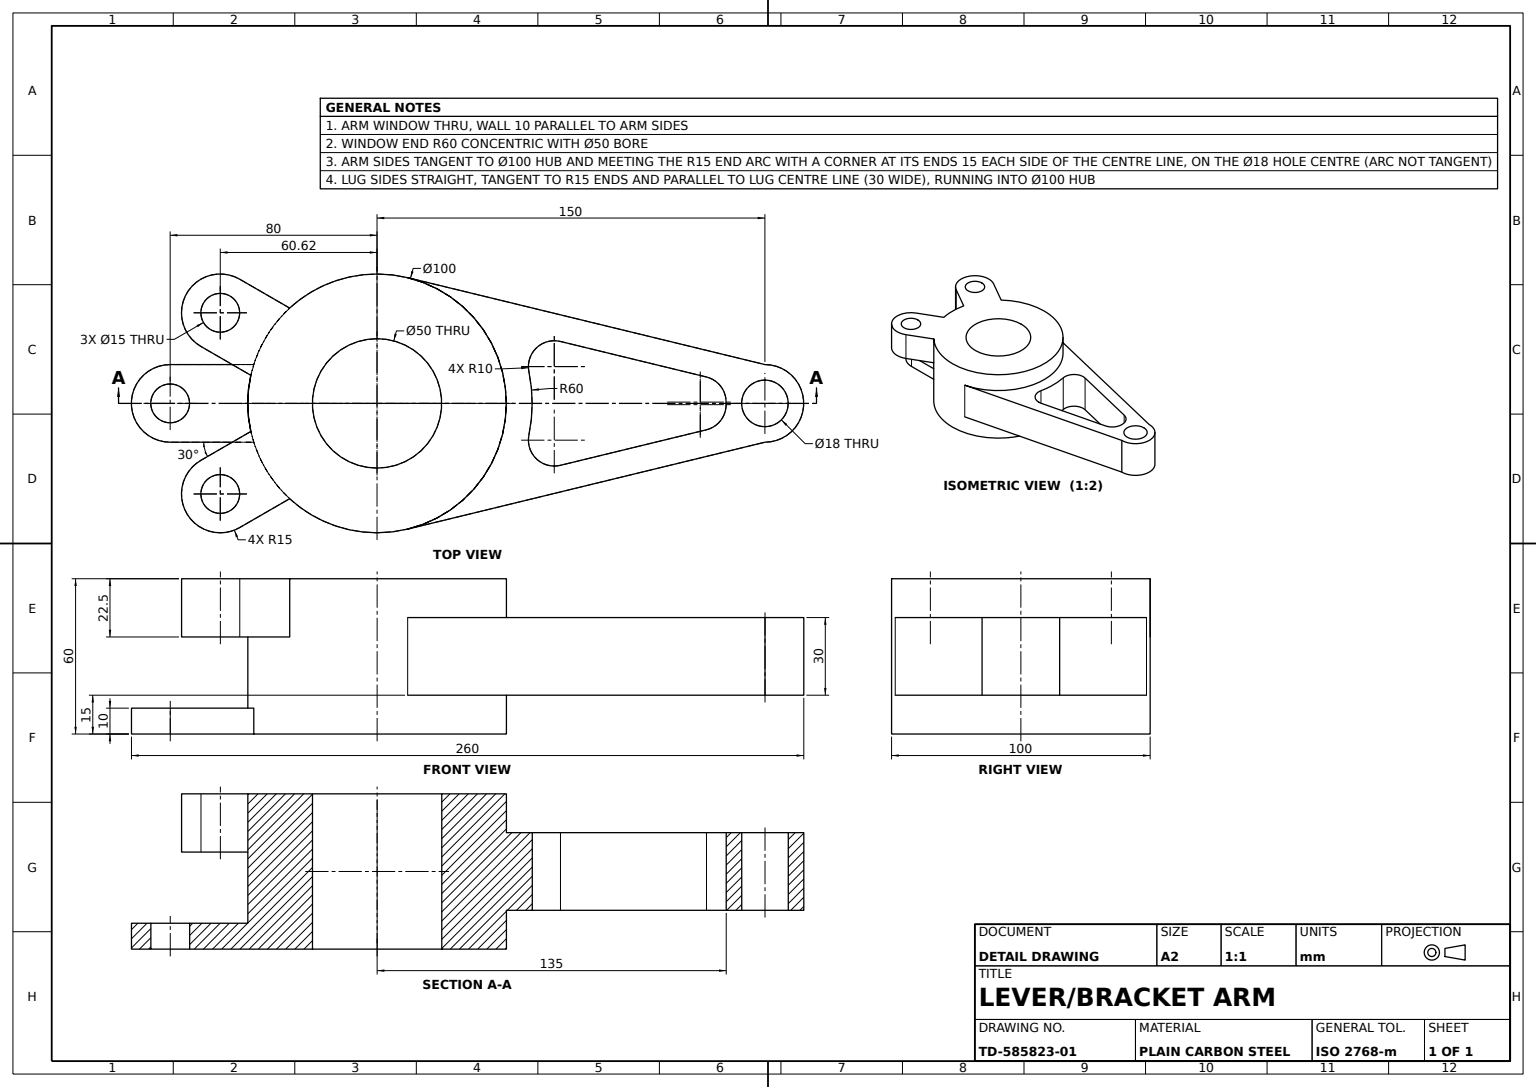
SolidWorks part; units mm, degrees
material "Plain Carbon Steel"
ref_plane "Front Plane" through (0, 0, 0) normal (0, 0, 1) x (1, 0, 0)
ref_plane "Top Plane" through (0, 0, 0) normal (0, 1, 0) x (1, 0, 0)
ref_plane "Right Plane" through (0, 0, 0) normal (1, 0, 0) x (0, 0, -1)
sketch "Hub Sketch" plane through (0, 0, 0) normal (0, 1, 0) x (1, 0, 0)
  circle A0 centre (0, 0) radius 25
  circle A1 centre (0, 0) radius 50
  dimension "D1" = 50
  dimension "D2" = 100
extrude "Hub Ø100 Bore Ø50" add sketch "Hub Sketch" along normal blind 60
ref_plane "Plane1" through (0, 30, 0) normal (0, 1, 0) x (1, 0, 0)
sketch "Lever Arm Sketch" plane through (0, 30, 0) normal (0, 1, 0) x (1, 0, 0)
  line L0 (0, 0) -> (150, 0) construction
  line L1 (11.8081, 48.5857) -> (150, 15)
  line L2 (11.8081, -48.5857) -> (150, -15)
  circle A0 centre (150, 0) radius 9
  arc A1 (150, -15) -> (150, 15) centre (150, 0) ccw
  circle A2 centre (0, 0) radius 50 construction
  arc A4 (11.8081, 48.5857) -> (11.8081, -48.5857) centre (0, 0) cw
  dimension "D1" = 18
  dimension "D2" = 30
  dimension "D3" = 150
extrude "Lever Arm" add sketch "Lever Arm Sketch" along normal mid plane 30
sketch "Arm Window Sketch" plane through (0, 45, 0) normal (0, 1, 0) x (1, 0, 0)
  line L2 (147.6384, 5.2829) -> (9.4465, 38.8685)
  line L3 (127.3665, 10.2097) -> (70.903, 23.9324)
  line L5 (9.4465, -38.8685) -> (147.6384, -5.2829)
  line L6 (70.903, -23.9324) -> (127.3665, -10.2097)
  arc A0 (58.7498, -12.1845) -> (58.7498, 12.1845) centre (0, 0) ccw
  arc A1 (70.903, 23.9324) -> (58.7498, 12.1845) centre (68.5414, 14.2152) ccw
  arc A2 (58.7498, -12.1845) -> (70.903, -23.9324) centre (68.5414, -14.2152) ccw
  arc A3 (135.0029, 0.2955) -> (135.0029, -0.2955) centre (150, 0) ccw
  arc A4 (135.0029, 0.2955) -> (127.3665, 10.2097) centre (125.0049, 0.4925) ccw
  arc A5 (127.3665, -10.2097) -> (135.0029, -0.2955) centre (125.0049, -0.4925) ccw
  dimension "D1" = 120
  dimension "D4" = 10
  dimension "D5" = 10
  dimension "D6" = 30
  dimension "D7" = 10
  dimension "D8" = 10
  dimension "D2" = 10
  dimension "D3" = 10
extrude "Arm Lightening Window" cut sketch "Arm Window Sketch" against normal through all
ref_plane "Plane2" through (0, 60, 0) normal (0, 1, 0) x (1, 0, 0)
sketch "Ear A Sketch" plane through (0, 60, 0) normal (0, 1, 0) x (1, 0, 0)
  line L0 (0, 0) -> (-106.1022, 0) construction
  line L1 (0, 0) -> (0, -99.3299) construction
  line L3 (-48.7701, -10.8369) -> (-68.1218, -22.0096)
  line L4 (-33.645, -36.7454) -> (-53.1218, -47.9904)
  arc A0 (-68.1218, -22.0096) -> (-53.1218, -47.9904) centre (-60.6218, -35) ccw
  circle A1 centre (-60.6218, -35) radius 7.5
  arc A2 (-48.7701, -10.8369) -> (-33.645, -36.7454) centre (-0.1675, 0.1675) ccw
  point P7 (-7.5, 12.9904)
  point P9 (7.5, -12.9904)
  dimension "D2" = 30
  dimension "D3" = 15
  dimension "D7" = 48.7701
  dimension "D1" = 49.8328
  dimension "D4" = 70
  dimension "D5" = 0.1675
  dimension "D6" = 33.645
  dimension "D8" = 53.1218
  dimension "D9" = 60.6218
extrude "Mounting Ear A" add sketch "Ear A Sketch" against normal blind 22.5
sketch "Ear B Sketch" plane through (0, 60, 0) normal (0, 1, 0) x (1, 0, 0)
  line L0 (0, 0) -> (-112.1045, 0) construction
  line L2 (-33.8068, 36.8389) -> (-53.1218, 47.9904)
  line L3 (-48.8068, 10.8581) -> (-68.1218, 22.0096)
  circle A0 centre (-60.6218, 35) radius 7.5
  arc A1 (-53.1218, 47.9904) -> (-68.1218, 22.0096) centre (-60.6218, 35) ccw
  arc A2 (-33.8068, 36.8389) -> (-48.8068, 10.8581) centre (0, 0) ccw
  arc A3 (-33.8068, -36.8389) -> (-48.8068, -10.8581) centre (0, 0) ccw construction
  point P6 (7.5, 12.9904)
  point P8 (-7.5, -12.9904)
  dimension "D3" = 30
  dimension "D4" = 15
  dimension "D1" = 7.5
  dimension "D2" = 70
  dimension "D5" = 15
extrude "Mounting Ear B" add sketch "Ear B Sketch" against normal blind 22.5
ref_plane "Plane4" through (0, 0, 0) normal (0, 1, 0) x (1, 0, 0)
sketch "Arm Web Sketch" plane through (0, 0, 0) normal (0, 1, 0) x (1, 0, 0)
  line L0 (-80, 15) -> (-50.6612, 15)
  line L1 (-80, -15) -> (-43.0437, -15)
  line L2 (-43.0437, -15) -> (-43.0437, 15)
  line L3 (-43.0437, 15) -> (-50.6612, 15)
  circle A0 centre (-80, 0) radius 7.5
  arc A1 (-80, 15) -> (-80, -15) centre (-80, 0) ccw
  dimension "D1" = 30
  dimension "D2" = 15
  dimension "D3" = 80
  dimension "D4" = 29.3388
  dimension "D5" = 36.9563
extrude "Arm Web 10mm" add sketch "Arm Web Sketch" along normal blind 10
